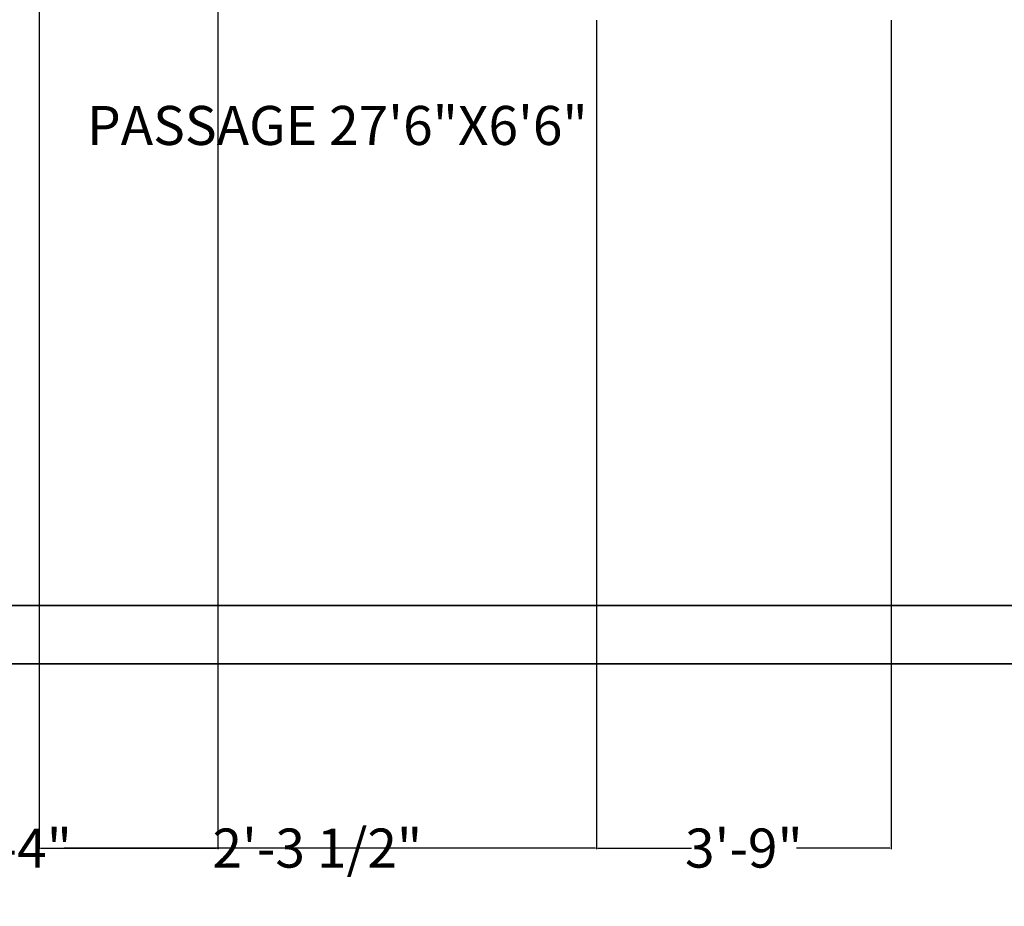
# Model space of a CAD drawing. Units: inches. Extents: x -26 to 575, y -18 to 513.
# Tile 2 of 28: x 122 to 274, y -18 to 119. Entities that reach past the tile are written whole.
import ezdxf

# ---------------------------------------------------------------- set-up
doc = ezdxf.new("R2010")
doc.units = ezdxf.units.IN
doc.header["$MEASUREMENT"] = 0
for name, color, linetype, lineweight in [('A-ANNO-DIMS', 2, 'Continuous', 18), ('A-AREA-IDEN', 7, 'Continuous', 18), ('A-WALL', 7, 'Continuous', 35)]:
    doc.layers.add(name, color=color, linetype=linetype, lineweight=lineweight)
doc.styles.get("Standard").update_dxf_attribs({"font": 'arial.ttf', "height": 6})
doc.dimstyles.get("Standard").update_dxf_attribs({"dimtxt": 6, "dimasz": 0.18, "dimexe": 0.18, "dimexo": 0.0625, "dimgap": 0.09, "dimtad": 0, "dimtih": 1, "dimtoh": 1, "dimzin": 0, "dimdsep": 46, "dimlunit": 3, "dimtxsty": 'Standard', "dimcen": 0.09, "dimadec": 0, "dimazin": 0, "dimtfac": 1, "dimtofl": 0, "dimtmove": 0, "dimatfit": 3, "dimfxl": 1, "dimtolj": 1, "dimtzin": 0, "dimarcsym": 0})

# ---------------------------------------------------------------- blocks, each defined once
blk = doc.blocks.new('*D29')
at = {"layer": 'A-ANNO-DIMS', "color": 0, "lineweight": -2, "transparency": 16777216}
for p, q in [((125.35, 466.45), (125.35, -8.97)), ((152.78, 466.45), (152.78, -8.97)), ((125.53, -8.79), (152.6, -8.79)), ((152.78, -8.79), (152.96, -8.79))]:
    blk.add_line(p, q, dxfattribs=at)
at = {"layer": 'A-ANNO-DIMS', "color": 0, "transparency": 16777216}
for points in [[(125.53, -8.76), (125.53, -8.82), (125.35, -8.79)], [(152.6, -8.76), (152.6, -8.82), (152.78, -8.79)]]:
    blk.add_solid(points, dxfattribs=at)
at = {"layer": 'Defpoints', "color": 0, "transparency": 16777216}
for p in [(125.35, 466.51), (152.78, 466.51), (152.78, -8.79)]:
    blk.add_point(p, dxfattribs=at)
at = {"layer": 'A-ANNO-DIMS', "color": 0, "transparency": 16777216, "insert": (168.07, -8.79), "char_height": 6, "attachment_point": 5}
blk.add_mtext('\\A1;2\'-3 1/2"', dxfattribs=at)
blk = doc.blocks.new('*D39')
at = {"layer": 'A-ANNO-DIMS', "color": 0, "lineweight": -2, "transparency": 16777216}
for p, q in [((210.97, 118.45), (210.97, -8.97)), ((256.19, 118.45), (256.19, -8.97)), ((211.15, -8.79), (225.52, -8.79)), ((256.01, -8.79), (241.64, -8.79))]:
    blk.add_line(p, q, dxfattribs=at)
at = {"layer": 'A-ANNO-DIMS', "color": 0, "transparency": 16777216}
for points in [[(211.15, -8.76), (211.15, -8.82), (210.97, -8.79)], [(256.01, -8.76), (256.01, -8.82), (256.19, -8.79)]]:
    blk.add_solid(points, dxfattribs=at)
at = {"layer": 'Defpoints', "color": 0, "transparency": 16777216}
for p in [(210.97, 118.51), (256.19, 118.51), (256.19, -8.79)]:
    blk.add_point(p, dxfattribs=at)
at = {"layer": 'A-ANNO-DIMS', "color": 0, "transparency": 16777216, "insert": (233.58, -8.79), "char_height": 6, "attachment_point": 5}
blk.add_mtext('\\A1;3\'-9"', dxfattribs=at)
blk = doc.blocks.new('*D40')
at = {"layer": 'A-ANNO-DIMS', "color": 0, "lineweight": -2, "transparency": 16777216}
for p, q in [((27.18, 118.45), (27.18, -8.97)), ((210.97, 118.45), (210.97, -8.97)), ((27.36, -8.79), (108.96, -8.79)), ((210.79, -8.79), (129.19, -8.79))]:
    blk.add_line(p, q, dxfattribs=at)
at = {"layer": 'A-ANNO-DIMS', "color": 0, "transparency": 16777216}
for points in [[(27.36, -8.76), (27.36, -8.82), (27.18, -8.79)], [(210.79, -8.76), (210.79, -8.82), (210.97, -8.79)]]:
    blk.add_solid(points, dxfattribs=at)
at = {"layer": 'Defpoints', "color": 0, "transparency": 16777216}
for p in [(27.18, 118.51), (210.97, 118.51), (27.18, -8.79)]:
    blk.add_point(p, dxfattribs=at)
at = {"layer": 'A-ANNO-DIMS', "color": 0, "transparency": 16777216, "insert": (119.07, -8.79), "char_height": 6, "attachment_point": 5}
blk.add_mtext('\\A1;15\'-4"', dxfattribs=at)

msp = doc.modelspace()

# ---------------------------------------------------------------- linework, layer by layer
at = {"layer": 'A-WALL'}
msp.add_line((27.177, 28.508), (513.177, 28.508), dxfattribs=at)
msp.add_lwpolyline([(18.177, 19.508), (522.177, 19.508), (522.177, 475.508), (18.177, 475.508)], close=True, dxfattribs=at)

# ---------------------------------------------------------------- texts
at = {"layer": 'A-AREA-IDEN'}
msp.add_text('PASSAGE 27\'6"X6\'6"', height=6, rotation=0.00167, dxfattribs=at).set_placement((132.69, 99.252))

# ---------------------------------------------------------------- dimensions: what is measured, and where the dimension line sits
at = {"layer": 'A-ANNO-DIMS'}
for base, p1, p2, picture, middle in [((152.784, -8.792), (125.349, 466.508), (152.784, 466.508), '*D29', (168.07, -8.792)), ((27.177, -8.792), (210.969, 118.508), (27.177, 118.508), '*D40', (119.073, -8.792)), ((256.192, -8.792), (210.969, 118.508), (256.192, 118.508), '*D39', (233.581, -8.792))]:
    dim = msp.add_linear_dim(base=base, p1=p1, p2=p2, dimstyle='Standard', override={"dimdec": 1, "dimlfac": 1, "dimrnd": 0, "dimzin": 1, "dimdsep": 46, "dimlunit": 4, "dimfrac": 2}, dxfattribs=at)
    dim.commit()
    dim.dimension.update_dxf_attribs({"geometry": picture, "text_midpoint": middle})

doc.saveas('drawing.dxf')
